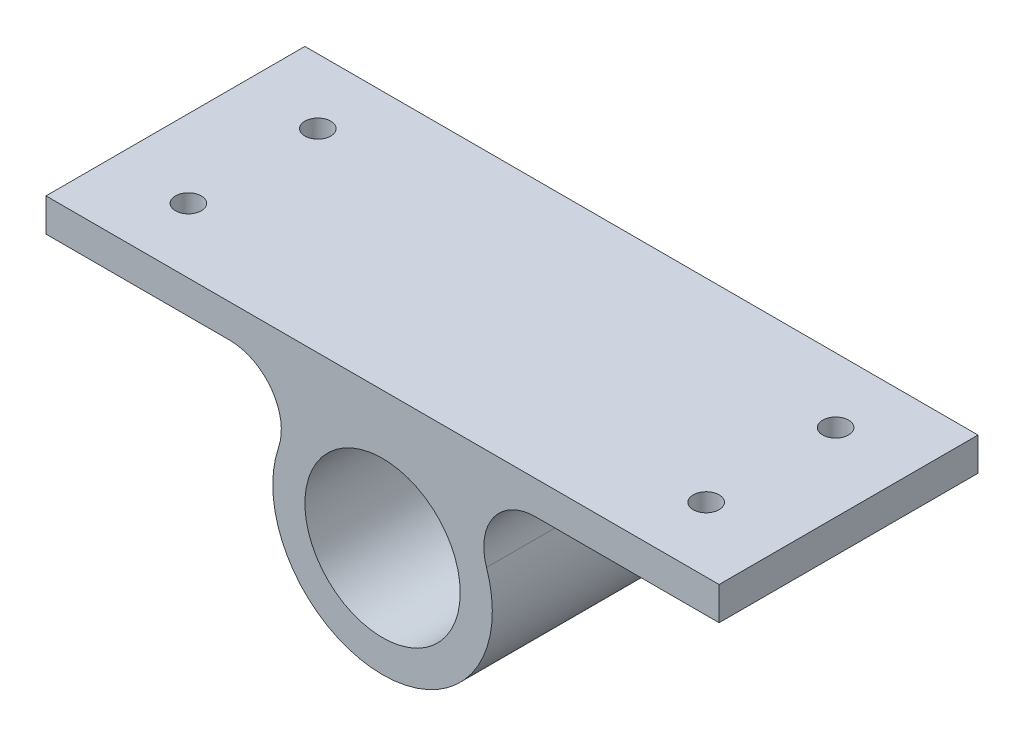
SolidWorks part; units mm, degrees
material "Plain Carbon Steel"
ref_plane "Front Plane" through (0, 0, 0) normal (0, 0, 1) x (1, 0, 0)
ref_plane "Top Plane" through (0, 0, 0) normal (0, 1, 0) x (1, 0, 0)
ref_plane "Right Plane" through (0, 0, 0) normal (1, 0, 0) x (0, 0, -1)
sketch "Pivot Bracket Profile" plane through (0, 0, 0) normal (0, 0, 1) x (1, 0, 0)
  line L0 (147.7701, 100) -> (325, 100)
  line L1 (-325, 132) -> (325, 132)
  line L2 (-325, 132) -> (-325, 100)
  line L3 (-325, 100) -> (-147.7701, 100)
  line L4 (325, 132) -> (325, 100)
  line L5 (-325, 132) -> (325, 100) construction
  line L6 (-325, 100) -> (325, 132) construction
  circle A0 centre (0, 0) radius 75
  arc A1 (-100.4079, 33.9744) -> (100.4079, 33.9744) centre (0, 0) ccw
  arc A2 (-100.4079, 33.9744) -> (-147.7701, 100) centre (-147.7701, 50) ccw
  arc A3 (147.7701, 100) -> (100.4079, 33.9744) centre (147.7701, 50) ccw
  point P4 (0, 116)
  dimension "D1" = 150
  dimension "D2" = 212
  dimension "D6" = 100
  dimension "D7" = 100
  dimension "D3" = 325
  dimension "D4" = 132
  dimension "D5" = 32
extrude "Pivot Bracket Body" add sketch "Pivot Bracket Profile" along normal mid plane 250
sketch "Mounting Holes Sketch" plane through (0, 132, 0) normal (0, 1, 0) x (1, 0, 0)
  line L0 (325, 125) -> (-325, 125) construction
  line L1 (-325, -125) -> (-325, 125) construction
  line L2 (0, -130.9) -> (0, 130.9) construction
  circle A0 centre (-250, 62.5) radius 12.5
  circle A1 centre (-250, -62.5) radius 12.5
  circle A2 centre (250, -62.5) radius 12.5
  circle A3 centre (250, 62.5) radius 12.5
  dimension "D1" = 25
  dimension "D2" = 25
  dimension "D3" = 62.5
  dimension "D4" = 125
  dimension "D5" = 75
extrude "Mounting Holes 4x" cut sketch "Mounting Holes Sketch" against normal mid plane 250
